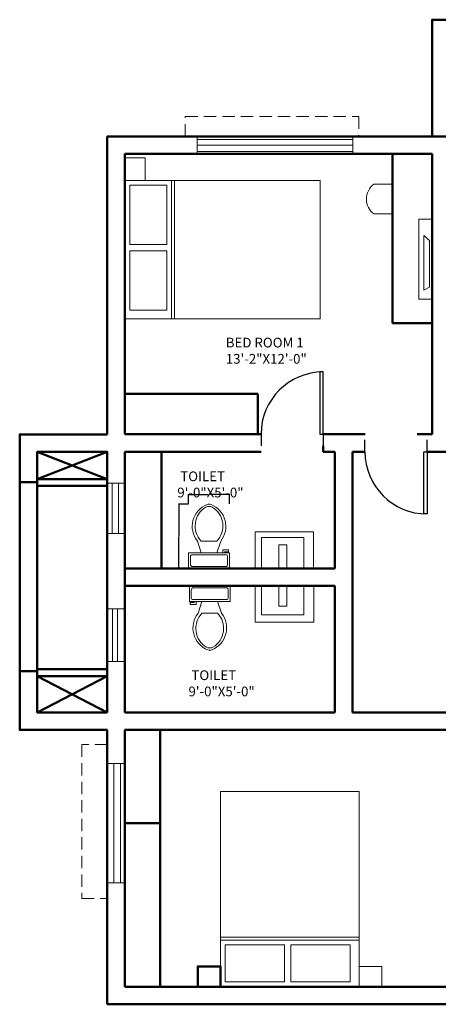
# Model space of a CAD drawing. Units: inches. Extents: x -105 to 1531, y -656 to 2003.
# Tile 3 of 6: x 338 to 553, y 594 to 1100. Entities that reach past the tile are written whole.
import ezdxf

# ---------------------------------------------------------------- set-up
doc = ezdxf.new("R2010")
doc.units = ezdxf.units.IN
doc.header["$MEASUREMENT"] = 0
doc.linetypes.add('DASHED', pattern=[19.05, 12.7, -6.35])
for name, color, linetype, lineweight in [('A-ANNO-DIMS', 2, 'Continuous', 18), ('A-AREA-IDEN', 7, 'Continuous', 25), ('A-DOOR', 3, 'Continuous', 25), ('A-FLOR-FIXT', 9, 'Continuous', 18), ('A-FLOR-OVHD', 8, 'DASHED', 18), ('A-FURN', 8, 'Continuous', 18), ('A-GLAZ', 4, 'Continuous', 18), ('A-WALL', 7, 'Continuous', 50)]:
    doc.layers.add(name, color=color, linetype=linetype, lineweight=lineweight)
doc.styles.get("Standard").update_dxf_attribs({"font": 'arial.ttf'})
doc.dimstyles.get("Standard").update_dxf_attribs({"dimtxt": 0.18, "dimasz": 0.18, "dimexe": 0.18, "dimexo": 0.0625, "dimgap": 0.09, "dimtad": 0, "dimtih": 1, "dimtoh": 1, "dimdec": 0, "dimzin": 0, "dimdsep": 46, "dimlunit": 3, "dimtxsty": 'Standard', "dimcen": 0.09, "dimadec": 0, "dimazin": 0, "dimtfac": 1, "dimtdec": 0, "dimtofl": 0, "dimtmove": 0, "dimatfit": 3, "dimfxl": 1, "dimtolj": 1, "dimtzin": 0, "dimarcsym": 0})

# ---------------------------------------------------------------- blocks, each defined once
blk = doc.blocks.new('*U13')
for p, q in [((-32, 0), (-32, -6)), ((0, 0), (0, -6))]:
    blk.add_line(p, q)
blk.add_lwpolyline([(0, 0), (0, 32), (-1.75, 32), (-1.75, 0)], close=True)
blk.add_arc((0, 0), 32, 90, 180)
blk = doc.blocks.new('*U14')
for p, q in [((-32, 0), (-32, 6)), ((0, 0), (0, 6))]:
    blk.add_line(p, q)
blk.add_lwpolyline([(0, 0), (0, -32), (-1.75, -32), (-1.75, 0)], close=True)
blk.add_arc((0, 0), 32, 180, 270)
blk = doc.blocks.new('Toilet - top')
for p, q in [((9.5, -6), (9.5, -2)), ((-10, -8.5), (-8, -8.5)), ((-10, -9.5), (-10, -8.5)), ((-7, -9.5), (-10, -9.5)), ((-8, -8.5), (-8, -8)), ((-7, -8), (-7, -9.5)), ((-4, -8), (-6, -14)), ((4, -8), (6, -14)), ((4, -14), (-4, -14))]:
    blk.add_line(p, q)
blk.add_lwpolyline([(10.5, -8), (10.5, 0), (-10.5, 0), (-10.5, -8)], close=True)
for points in [[(-9.5, -2), (-9.5, -6)], [(8.5, -1), (-8.5, -1)], [(-8.5, -7), (8.5, -7)]]:
    blk.add_lwpolyline(points)
for centre, radius, start, end in [((-8.62, -1.88), 0.884, 81.8699, 188.1301), ((8.62, -1.88), 0.884, 351.8699, 98.1301), ((-8.62, -6.12), 0.884, 171.8699, 278.1301), ((8.62, -6.12), 0.884, 261.8699, 8.1301), ((3.52, -21.58), 12.17, 141.4691, 247.9714), ((4.2, -21.82), 11.33, 136.3677, 238.9468), ((-3.52, -21.58), 12.17, 292.0284, 38.5307), ((-4.2, -21.82), 11.33, 301.053, 43.6321), ((0, -27.88), 4, 245.7318, 294.2682), ((0, -29), 4, 254.8605, 285.1395)]:
    blk.add_arc(centre, radius, start, end)
blk = doc.blocks.new('FURN-SIDE-TABLE')
for p, q in [((13.4, 15.25), (3.8, 15.25)), ((13.4, 0), (13.4, 15.25)), ((3.8, 0), (13.4, 0))]:
    blk.add_line(p, q)
blk.add_arc((9.55, 7.62), 9.55, 127.0288, 232.9712)
blk = doc.blocks.new('*D27')
at = {"layer": 'A-ANNO-DIMS', "color": 0, "lineweight": -2, "transparency": 16777216}
for p, q in [((424.76, 850.61), (419.69, 850.61)), ((419.87, 850.43), (419.87, 834.27)), ((419.87, 817.75), (419.87, 833.91)), ((424.76, 817.57), (419.69, 817.57))]:
    blk.add_line(p, q, dxfattribs=at)
at = {"layer": 'A-ANNO-DIMS', "color": 0, "transparency": 16777216}
for points in [[(419.84, 850.43), (419.9, 850.43), (419.87, 850.61)], [(419.84, 817.75), (419.9, 817.75), (419.87, 817.57)]]:
    blk.add_solid(points, dxfattribs=at)
at = {"layer": 'Defpoints', "color": 0, "transparency": 16777216}
for p in [(424.83, 850.61), (419.87, 817.57), (424.83, 817.57)]:
    blk.add_point(p, dxfattribs=at)
at = {"layer": 'A-ANNO-DIMS', "color": 0, "transparency": 16777216, "insert": (419.87, 834.09), "char_height": 0.18, "attachment_point": 5}
blk.add_mtext('\\A1;WC 33 TYP.', dxfattribs=at)
blk = doc.blocks.new('*D28')
at = {"layer": 'A-ANNO-DIMS', "color": 0, "lineweight": -2, "transparency": 16777216}
for p, q in [((424.83, 850.68), (424.83, 855.75)), ((425.01, 855.57), (434.8, 855.57)), ((445.65, 855.57), (435.86, 855.57)), ((445.83, 850.68), (445.83, 855.75))]:
    blk.add_line(p, q, dxfattribs=at)
at = {"layer": 'A-ANNO-DIMS', "color": 0, "transparency": 16777216}
for points in [[(425.01, 855.6), (425.01, 855.54), (424.83, 855.57)], [(445.65, 855.6), (445.65, 855.54), (445.83, 855.57)]]:
    blk.add_solid(points, dxfattribs=at)
at = {"layer": 'Defpoints', "color": 0, "transparency": 16777216}
for p in [(424.83, 855.57), (424.83, 850.61), (445.83, 850.61)]:
    blk.add_point(p, dxfattribs=at)
at = {"layer": 'A-ANNO-DIMS', "color": 0, "transparency": 16777216, "insert": (435.33, 855.57), "char_height": 0.18, "attachment_point": 5}
blk.add_mtext('\\A1;21 TYP.', dxfattribs=at)

msp = doc.modelspace()

# ---------------------------------------------------------------- linework, layer by layer
at = {"layer": 'A-FLOR-FIXT'}
for points in [[(459.08, 817.57), (489.07, 817.57), (489.07, 836.37), (459.08, 836.37)], [(462.34, 817.57), (483.97, 817.57), (483.97, 833.41), (462.34, 833.41)], [(471.12, 817.57), (475.3, 817.57), (475.3, 829.74), (471.12, 829.74)]]:
    msp.add_lwpolyline(points, close=True, dxfattribs=at)
for points in [[(459.08, 817.57), (489.15, 817.57)], [(462.34, 817.57), (484.06, 817.57)], [(471.12, 817.57), (475.39, 817.57)], [(489.15, 808.57), (489.15, 790.01), (459.08, 790.01), (459.08, 808.57)], [(484.06, 808.57), (484.06, 793.65), (462.34, 793.65), (462.34, 808.57)], [(475.39, 808.57), (475.39, 798.23), (471.12, 798.23), (471.12, 808.57)]]:
    msp.add_lwpolyline(points, dxfattribs=at)
at = {"layer": 'A-FLOR-OVHD', "ltscale": 0.5}
for p, q in [((423.13, 1039.57), (423.13, 1049.83)), ((423.13, 1049.83), (512.37, 1049.83)), ((512.37, 1049.83), (512.37, 1039.57)), ((383, 727.03), (369.92, 727.03)), ((369.92, 727.03), (369.92, 647.9)), ((369.92, 647.9), (383, 647.9))]:
    msp.add_line(p, q, dxfattribs=at)
at = {"layer": 'A-FURN'}
for p, q in [((416.04, 1016.97), (416.04, 945.79)), ((417.55, 945.79), (417.55, 1016.97)), ((545.81, 960.57), (545.81, 988.65)), ((545.81, 988.65), (548.7, 986.16)), ((548.7, 986.16), (548.7, 962.04)), ((545.81, 960.57), (548.7, 962.04)), ((416.04, 945.79), (417.55, 945.79)), ((512.41, 628.11), (441.23, 628.11)), ((512.41, 626.61), (512.41, 628.11)), ((441.23, 626.61), (512.41, 626.61))]:
    msp.add_line(p, q, dxfattribs=at)
for points in [[(392, 1028.66), (402.46, 1028.66), (402.46, 1016.97), (392, 1016.97)], [(392, 1016.97), (492.4, 1016.97), (492.4, 945.79), (392, 945.79)], [(394.55, 1014.51), (413.55, 1014.51), (413.55, 984.03), (394.55, 984.03)], [(550, 997.01), (543.16, 997.01), (543.16, 955.97), (550, 955.97)], [(394.55, 980.84), (413.55, 980.84), (413.55, 950.36), (394.55, 950.36)], [(441.23, 602.57), (441.23, 702.97), (512.41, 702.97), (512.41, 602.57)], [(443.69, 605.12), (443.69, 624.12), (474.17, 624.12), (474.17, 605.12)], [(477.36, 605.12), (477.36, 624.12), (507.84, 624.12), (507.84, 605.12)], [(512.41, 602.57), (512.41, 613.02), (524.1, 613.02), (524.1, 602.57)]]:
    msp.add_lwpolyline(points, close=True, dxfattribs=at)
at = {"layer": 'A-GLAZ'}
for p, q in [((429.26, 1030.57), (429.26, 1039.57)), ((429.26, 1039.57), (509.15, 1039.57)), ((429.26, 1035.07), (429.26, 1038)), ((429.26, 1038), (509.15, 1038)), ((509.15, 1039.57), (509.15, 1030.57)), ((509.15, 1035.07), (429.26, 1035.07)), ((509.15, 1031.87), (509.15, 1035.07)), ((429.26, 1030.57), (429.26, 1031.87)), ((429.26, 1031.87), (509.15, 1031.87)), ((509.15, 1030.57), (429.26, 1030.57)), ((383, 861.33), (392, 861.33)), ((388.87, 861.33), (385.59, 861.33)), ((385.59, 861.33), (385.59, 835.55)), ((388.87, 835.55), (388.87, 861.33)), ((392, 861.33), (392, 835.55)), ((392, 835.55), (383, 835.55)), ((383, 796.84), (392, 796.84)), ((385.76, 769.73), (385.76, 796.84)), ((385.76, 796.84), (388.31, 796.84)), ((388.31, 796.84), (388.31, 769.73)), ((392, 796.84), (392, 769.73)), ((392, 769.73), (383, 769.73)), ((383, 769.73), (385.76, 769.73)), ((383, 717.4), (392, 717.4)), ((383, 655.99), (383, 717.4)), ((383, 717.4), (386.32, 717.4)), ((386.32, 717.4), (386.32, 655.99)), ((389.9, 655.99), (389.9, 717.4)), ((392, 717.4), (392, 655.99)), ((392, 655.99), (383, 655.99)), ((389.9, 655.99), (392, 655.99))]:
    msp.add_line(p, q, dxfattribs=at)
at = {"layer": 'A-WALL'}
for p, q in [((559, 1039.57), (383, 1039.57)), ((383, 886.44), (383, 1039.57)), ((550, 1039.57), (559, 1039.57)), ((550, 1030.57), (392, 1030.57)), ((392, 886.57), (392, 1030.57)), ((529.6, 1030.57), (529.6, 943.6)), ((550, 924.12), (550, 1030.57)), ((529.6, 943.6), (550, 943.6)), ((550, 892.27), (550, 928.27)), ((392, 907.36), (392, 907.36)), ((392, 907.36), (460.39, 907.36)), ((460.39, 907.36), (460.39, 886.57)), ((550, 886.57), (550, 892.27)), ((462.05, 886.57), (392, 886.57)), ((515.56, 886.57), (494.05, 886.57)), ((547.42, 886.57), (542.23, 886.57)), ((550, 886.57), (547.42, 886.57)), ((494.05, 880.57), (494.05, 877.57)), ((383, 877.44), (347, 877.44)), ((347, 863.38), (383, 877.44)), ((383, 863.38), (347, 877.44)), ((383, 743.57), (383, 877.44)), ((383, 877.44), (383, 863.38)), ((392, 817.57), (392, 877.57)), ((462.19, 877.57), (392, 877.57)), ((410.81, 877.57), (410.81, 817.57)), ((500, 877.57), (494.05, 877.57)), ((500, 817.57), (500, 877.57)), ((509, 743.57), (509, 877.57)), ((515.42, 877.57), (509, 877.57)), ((559, 877.57), (547.42, 877.57)), ((347, 861.84), (338, 861.84)), ((338, 861.84), (338, 764.76)), ((347, 863.38), (383, 863.38)), ((347, 860.03), (347, 863.38)), ((383, 863.38), (383, 860.03)), ((383, 860.03), (347, 860.03)), ((500, 817.57), (392, 817.57)), ((500, 808.57), (392, 808.57)), ((392, 743.57), (392, 808.57)), ((500, 743.57), (500, 808.57)), ((338, 764.76), (347, 764.76)), ((383, 765.72), (347, 765.72)), ((347, 765.72), (347, 762.15)), ((383, 762.15), (383, 765.72)), ((347, 762.15), (383, 762.15)), ((347, 762.15), (383, 743.57)), ((383, 762.15), (347, 743.57)), ((500, 743.57), (392, 743.57)), ((648, 743.57), (509, 743.57)), ((383, 593.57), (383, 734.57)), ((564, 734.57), (392, 734.57)), ((392, 602.57), (392, 734.57)), ((410.12, 734.57), (410.12, 602.57)), ((392, 686.69), (410.12, 686.69)), ((564, 602.57), (392, 602.57)), ((564, 593.57), (383, 593.57)), ((383, 593.57), (383, 593.57))]:
    msp.add_line(p, q, dxfattribs=at)
for points in [[(700, 1039.57), (700, 1099.57), (550, 1099.57), (550, 1039.57)], [(550, 1030.57), (550, 1009.57)], [(383, 734.57), (338, 734.57), (338, 886.44), (383, 886.44)], [(392, 877.57), (392, 743.57)]]:
    msp.add_lwpolyline(points, dxfattribs=at)
for points in [[(383, 743.57), (347, 743.57), (347, 877.44), (383, 877.44)], [(392, 734.57), (392, 734.57)], [(429.54, 602.57), (429.54, 613.02), (441.23, 613.02), (441.23, 602.57)]]:
    msp.add_lwpolyline(points, close=True, dxfattribs=at)

# ---------------------------------------------------------------- block references
at = {"layer": 'A-DOOR'}
for name, p in [('*U13', (494.05, 886.57)), ('*U14', (547.42, 877.57))]:
    msp.add_blockref(name, p, dxfattribs=at)
at = {"layer": 'A-FLOR-FIXT', "rotation": 180}
msp.add_blockref('Toilet - top', (435.33, 817.57), dxfattribs=at)
at = {"layer": 'A-FLOR-FIXT'}
msp.add_blockref('Toilet - top', (435.7, 808.57), dxfattribs=at)
at = {"layer": 'A-FURN'}
msp.add_blockref('FURN-SIDE-TABLE', (516.2, 999.76), dxfattribs=at)

# ---------------------------------------------------------------- texts
at = {"layer": 'A-AREA-IDEN', "ltscale": 5, "char_height": 5, "attachment_point": 1}
for s, insert in [('BED ROOM 1\\P13\'-2"X12\'-0"', (443.94, 936.12)), (' TOILET  \\P9\'-0"X5\'-0"', (419.02, 867.4)), (' TOILET  \\P9\'-0"X5\'-0"', (424.75, 765.18))]:
    msp.add_mtext_dynamic_manual_height_columns(s, width=114.6643, gutter_width=1, heights=[0], dxfattribs=dict(at, insert=insert))

# ---------------------------------------------------------------- dimensions: what is measured, and where the dimension line sits
at = {"layer": 'A-ANNO-DIMS'}
for base, p1, p2, angle, text, picture, middle in [((424.83, 855.57), (445.83, 850.61), (424.83, 850.61), 180, '<> TYP.', '*D28', (435.33, 855.57)), ((419.87, 817.57), (424.83, 850.61), (424.83, 817.57), 270, 'WC <> TYP.', '*D27', (419.87, 834.09))]:
    dim = msp.add_linear_dim(base=base, p1=p1, p2=p2, angle=angle, text=text, dimstyle='Standard', override={"dimdec": 0, "dimlfac": 1, "dimrnd": 0, "dimzin": 0, "dimdsep": 46, "dimlunit": 2}, dxfattribs=at)
    dim.commit()
    dim.dimension.update_dxf_attribs({"geometry": picture, "text_midpoint": middle})

doc.saveas('drawing.dxf')
